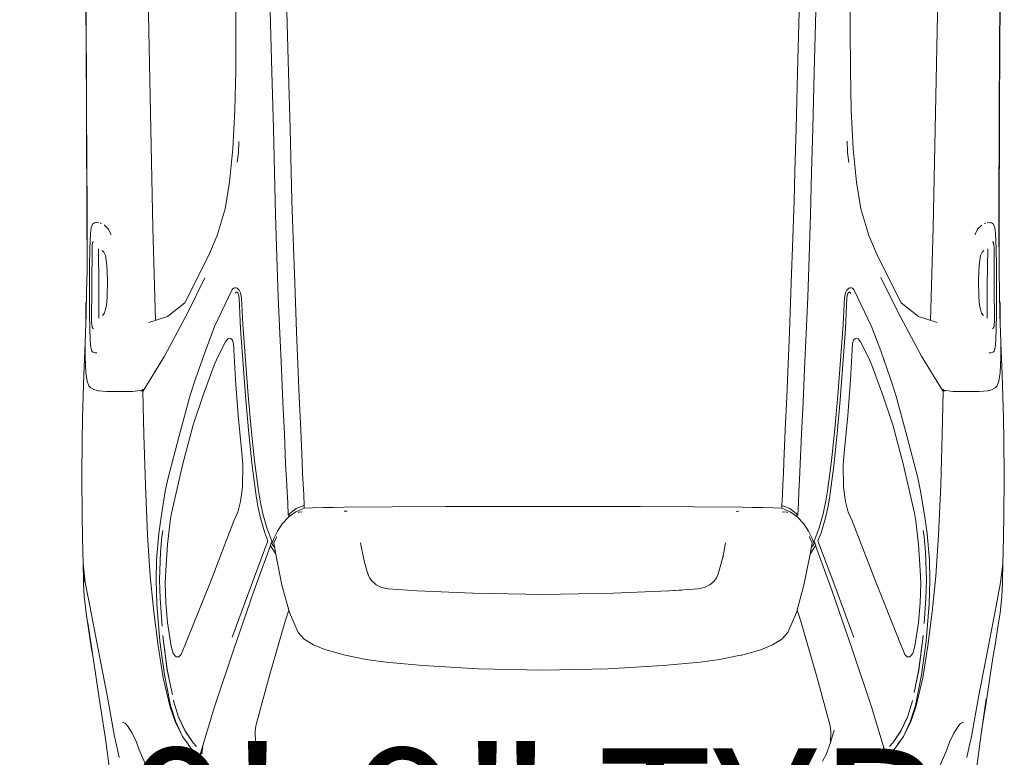
# Model space of a CAD drawing. Units: millimetres. Extents: x 595116 to 630915, y 909473 to 920225.
# Tile 115 of 134: x 629331 to 629393, y 919419 to 919466. Entities that reach past the tile are written whole.
import ezdxf

# ---------------------------------------------------------------- set-up
doc = ezdxf.new("R2010")
doc.units = ezdxf.units.MM
doc.layers.add('C-PRKG-VEHI', color=8, linetype='Continuous', lineweight=13)
doc.layers.add('Dimension', color=3, linetype='Continuous', lineweight=18)
doc.styles.get("Standard").update_dxf_attribs({"font": 'arial.ttf'})
doc.dimstyles.new('ISO-25', dxfattribs={"dimtxt": 9, "dimasz": 6, "dimexe": 1.25, "dimexo": 0.625, "dimtad": 1, "dimlunit": 4, "dimtxsty": 'Standard', "dimcen": 2.5, "dimadec": 0, "dimazin": 0, "dimtfac": 1, "dimtmove": 0, "dimatfit": 3, "dimfxl": 1, "dimarcsym": 0})

# ---------------------------------------------------------------- blocks, each defined once
blk = doc.blocks.new('A$C7ADB3080')
for p, q in [((2652.6, 1836.8), (2920.1, 1835.4)), ((2925, 1835.1), (2654.1, 1836.7)), ((3154.5, 1834.7), (2920.1, 1835.4)), ((2925, 1835.1), (3140.2, 1834.4)), ((3269.2, 1835.3), (3230.4, 1834.5)), ((3311.5, 1836.1), (3269.2, 1835.3)), ((3290.9, 1836.5), (3285.7, 1835.6)), ((3301, 1836.5), (3290.9, 1836.5)), ((3290.9, 1836.5), (3301, 1836.5)), ((3323.5, 1836.5), (3301, 1836.5)), ((3301, 1836.5), (3323.5, 1836.5)), ((3363.4, 1837.9), (3311.5, 1836.1)), ((3392, 1838.1), (3363.4, 1837.9)), ((3365.8, 1837.9), (3365.3, 1837.9)), ((3424.7, 1840.3), (3365.8, 1837.9)), ((3420.9, 1836.7), (3392, 1838.1)), ((3437.5, 1834.4), (3420.9, 1836.7)), ((3465.3, 1841.8), (3424.7, 1840.3)), ((3506.8, 1843), (3465.3, 1841.8)), ((3548.4, 1843.9), (3506.8, 1843)), ((3615.8, 1844.5), (3548.4, 1843.9)), ((3693.3, 1843.9), (3615.8, 1844.5)), ((3760.4, 1842.6), (3693.3, 1843.9)), ((3760.4, 1842.6), (3777.5, 1842)), ((3780.6, 1841.8), (3777.5, 1842)), ((3817.8, 1840.9), (3777.6, 1842)), ((3777.6, 1842), (3784.7, 1841.8)), ((3816.5, 1837.6), (3780.6, 1841.8)), ((3856.8, 1830), (3816.5, 1837.6)), ((3842, 1840.1), (3817.8, 1840.9)), ((3873.8, 1836.4), (3842, 1840.1)), ((3896.2, 1832.9), (3873.8, 1836.4)), ((3138.8, 1818), (3139.2, 1820.6)), ((3138.8, 1816.6), (3138.9, 1817.6)), ((3139.2, 1812.5), (3138.8, 1816.6)), ((3141.5, 1824), (3139.2, 1820.6)), ((3140.2, 1834.4), (3154.5, 1834.3)), ((3155.1, 1834.3), (3141.2, 1834.3)), ((3141.2, 1834.3), (3141.2, 1834.3)), ((3148.6, 1826.5), (3141.5, 1824)), ((3158.6, 1827.8), (3148.6, 1826.5)), ((3154.5, 1834.7), (3189.7, 1834.5)), ((3167.6, 1834.3), (3155.1, 1834.3)), ((3173, 1828.6), (3158.6, 1827.8)), ((3167.2, 1834.3), (3179.8, 1834.4)), ((3173, 1828.6), (3189, 1829)), ((3175.3, 1823.4), (3174.9, 1821.4)), ((3175.3, 1823.4), (3176.5, 1824)), ((3177.6, 1824.3), (3176.5, 1824)), ((3180.9, 1824.9), (3177.6, 1824.3)), ((3179.8, 1834.4), (3189.8, 1834.5)), ((3185.7, 1825.1), (3180.9, 1824.9)), ((3257.4, 1825.6), (3185.7, 1825.1)), ((3189, 1829), (3218.8, 1829.6)), ((3189.7, 1834.5), (3230.4, 1834.5)), ((3218.8, 1829.6), (3249.2, 1829.8)), ((3249.2, 1829.8), (3278.5, 1830)), ((3325.3, 1825.8), (3257.4, 1825.6)), ((3278.5, 1830), (3294.3, 1829.9)), ((3294.3, 1829.9), (3309.6, 1829.8)), ((3309.6, 1829.8), (3338.2, 1829.4)), ((3330.2, 1825.6), (3325.3, 1825.8)), ((3334.3, 1825.1), (3330.2, 1825.6)), ((3336.4, 1824.3), (3334.3, 1825.1)), ((3334.5, 1825), (3335.7, 1824.9)), ((3335.7, 1824.9), (3337.6, 1824)), ((3337.6, 1824), (3336.4, 1824.3)), ((3337.6, 1824), (3338, 1821.8)), ((3359.1, 1828.7), (3338.2, 1829.4)), ((3368.6, 1828), (3359.1, 1828.7)), ((3376.8, 1826.8), (3368.6, 1828)), ((3380.5, 1825.5), (3376.8, 1826.8)), ((3382.5, 1823.5), (3380.5, 1825.5)), ((3383.7, 1819.1), (3382.5, 1823.5)), ((3384, 1816), (3383.7, 1819.1)), ((3445.8, 1830.9), (3437.5, 1834.4)), ((3445.8, 1830.9), (3449.9, 1827.1)), ((3449.9, 1827.1), (3453.1, 1821.8)), ((3453.1, 1821.8), (3454.9, 1815.7)), ((3938.8, 1813.9), (3856.8, 1830)), ((3896.2, 1832.9), (3937.3, 1826.5)), ((3937.3, 1826.5), (3958, 1823.1)), ((3958, 1823.1), (4042.4, 1810.1)), ((3139.6, 1808.8), (3139.6, 1809.6)), ((3140.7, 1807.1), (3139.6, 1808.8)), ((3143.9, 1801.9), (3143.8, 1801.9)), ((3151.3, 1793.8), (3143.9, 1801.9)), ((3187.9, 1813.2), (3257.6, 1812.5)), ((3194.7, 1802.6), (3191.3, 1806.1)), ((3200.5, 1799.8), (3194.7, 1802.6)), ((3218.3, 1797.4), (3200.5, 1799.8)), ((3257.6, 1812.5), (3318.7, 1812.5)), ((3301.9, 1799.5), (3294.9, 1797.7)), ((3309.3, 1801.6), (3301.9, 1799.5)), ((3313.6, 1805.2), (3309.3, 1801.6)), ((3454.9, 1815.7), (3455.1, 1815)), ((3455.1, 1815), (3455.4, 1813.2)), ((3455.4, 1813.2), (3456.9, 1797.4)), ((4032, 1795.9), (3938.8, 1813.9)), ((4110.6, 1799.9), (4035.1, 1810.4)), ((4035.2, 1810.4), (4035.1, 1810.4)), ((4042.4, 1810.1), (4096.4, 1801.8)), ((4202.8, 1787.5), (4110.6, 1799.9)), ((3160.5, 1789.8), (3151.3, 1793.8)), ((3161.6, 1789.6), (3160.5, 1789.8)), ((3247.2, 1796.1), (3218.3, 1797.4)), ((3278.4, 1796.4), (3247.2, 1796.1)), ((3294.9, 1797.7), (3278.4, 1796.4)), ((3456.9, 1797.4), (3456.9, 1768.6)), ((4106, 1782.7), (4032, 1795.9)), ((4125.1, 1778.5), (4106, 1782.7)), ((3456.9, 1768.6), (3456.9, 1748.3)), ((4080, 1765.6), (4079.5, 1767.9)), ((4081, 1763.4), (4079.8, 1766.2)), ((4082.5, 1761.6), (4081, 1763.4)), ((4086.1, 1758.5), (4082.5, 1761.6)), ((4145.5, 1773.8), (4125.1, 1778.5)), ((3454.3, 1729.9), (3456.9, 1748.3)), ((4099.9, 1749.3), (4086.1, 1758.5)), ((4116.9, 1741.3), (4099.9, 1749.3)), ((3456.6, 1729.3), (3390, 1688.5)), ((3455.3, 1729.9), (3452.5, 1730)), ((3452.6, 1726.9), (3455.5, 1729.2)), ((3455.3, 1729.2), (3455.3, 1733.4)), ((3455.3, 1728.5), (3455.3, 1729)), ((3537.8, 1727.6), (3456.6, 1729.3)), ((3632.9, 1724.7), (3537.8, 1727.6)), ((3726.9, 1720.6), (3632.9, 1724.7)), ((4131.6, 1736.2), (4116.9, 1741.3)), ((4180, 1714.9), (4131.6, 1736.2)), ((3148.3, 1710.7), (2594.2, 1721.7)), ((3323, 1705.8), (3148.3, 1710.7)), ((3327.1, 1717.9), (3315.3, 1682.8)), ((3804.6, 1715.3), (3726.9, 1720.6)), ((3871.4, 1708.8), (3804.6, 1715.3)), ((3935.4, 1700.8), (3871.4, 1708.8)), ((3390, 1688.5), (3307.9, 1644.8)), ((3644.1, 1687), (3619.1, 1681.8)), ((3619.1, 1681.8), (3644.1, 1687)), ((3689.1, 1694.4), (3644.1, 1687)), ((3644.1, 1687), (3689.1, 1694.4)), ((3724.3, 1699.5), (3689.1, 1694.4)), ((3689.1, 1694.4), (3724.3, 1699.5)), ((3718.4, 1692), (3730.4, 1693.4)), ((3774.5, 1703.9), (3724.3, 1699.5)), ((3724.3, 1699.5), (3774.5, 1703.9)), ((3730.4, 1693.4), (3759.2, 1696)), ((3759.2, 1696), (3811.2, 1697.9)), ((3812.3, 1704.6), (3774.5, 1703.9)), ((3774.5, 1703.9), (3812.3, 1704.6)), ((3793.1, 1686.4), (3817.7, 1687.2)), ((3817.7, 1687.2), (3793.1, 1686.4)), ((3811.2, 1697.9), (3846.5, 1697)), ((3856.9, 1703.3), (3812.3, 1704.6)), ((3812.3, 1704.6), (3856.9, 1703.3)), ((3817.7, 1687.2), (3854.8, 1686)), ((3854.8, 1686), (3817.7, 1687.2)), ((3846.5, 1697), (3893.4, 1693.5)), ((3926.7, 1697.5), (3856.9, 1703.3)), ((3856.9, 1703.3), (3926.7, 1697.5)), ((3916.3, 1691.8), (3917.5, 1691.7)), ((3979.7, 1683.5), (3917.3, 1691.7)), ((3917.5, 1691.7), (3981.3, 1683.4)), ((3990.3, 1688.8), (3926.7, 1697.5)), ((3926.7, 1697.5), (3990.3, 1688.8)), ((3995.6, 1690.9), (3935.4, 1700.8)), ((4048.1, 1677.1), (3990.3, 1688.8)), ((3990.3, 1688.8), (4048.1, 1677.1)), ((4050.7, 1678.1), (3995.6, 1690.9)), ((3315.3, 1682.8), (3289.8, 1650.3)), ((3619.1, 1681.8), (3540, 1661.1)), ((3540, 1661.1), (3619.1, 1681.8)), ((3592.6, 1654.4), (3685.5, 1675.3)), ((3685.5, 1675.3), (3592.6, 1654.4)), ((3685.5, 1675.3), (3701, 1677.9)), ((3701, 1677.9), (3685.5, 1675.3)), ((3701, 1677.9), (3744.9, 1682.9)), ((3744.9, 1682.9), (3701, 1677.9)), ((3744.9, 1682.9), (3793.1, 1686.4)), ((3793.1, 1686.4), (3744.9, 1682.9)), ((3854.8, 1686), (3891.3, 1682.8)), ((3891.3, 1682.8), (3854.8, 1686)), ((3891.3, 1682.8), (3936.2, 1676.3)), ((3936.2, 1676.3), (3891.3, 1682.8)), ((3936.2, 1676.3), (3950.2, 1672.4)), ((3950.2, 1672.4), (3936.2, 1676.3)), ((3950.2, 1672.4), (3956.1, 1666.6)), ((3956.1, 1666.6), (3950.2, 1672.4)), ((4004.3, 1678.6), (3979.7, 1683.5)), ((3981.3, 1683.4), (4023.5, 1674.8)), ((4010.7, 1677.4), (4004.3, 1678.6)), ((4038.4, 1671.7), (4039.3, 1671.5)), ((4039.3, 1671.5), (4069.8, 1662)), ((4078.8, 1667.3), (4048.1, 1677.1)), ((4048.1, 1677.1), (4078.8, 1667.3)), ((4050.7, 1678.1), (4080.1, 1667.8)), ((4050.7, 1678.1), (4050.7, 1678.1)), ((4080.1, 1667.8), (4050.7, 1678.1)), ((3289.8, 1650.3), (3201.4, 1606)), ((3540, 1661.1), (3463.8, 1640.1)), ((3463.8, 1640.1), (3540, 1661.1)), ((3519.3, 1634.8), (3592.6, 1654.4)), ((3592.6, 1654.4), (3519.3, 1634.8)), ((3951.6, 1657.2), (3925.2, 1646.4)), ((3925.2, 1646.4), (3951.6, 1657.2)), ((3956, 1661.6), (3951.6, 1657.2)), ((3951.6, 1657.2), (3956, 1661.6)), ((3956.1, 1666.6), (3956, 1661.6)), ((3956, 1661.6), (3956.1, 1666.6)), ((4095.5, 1649.7), (4069.3, 1662.1)), ((4069.8, 1662), (4096.4, 1649.5)), ((4106, 1654.5), (4078.8, 1667.3)), ((4078.8, 1667.3), (4106, 1654.5)), ((4080.1, 1667.8), (4106, 1654.5)), ((4106, 1654.5), (4080.1, 1667.8)), ((4117.9, 1634.7), (4095.5, 1649.7)), ((4096.4, 1649.5), (4118.4, 1634.8)), ((4121, 1644.1), (4106, 1654.5)), ((4106, 1654.5), (4120.9, 1644.2)), ((3307.9, 1644.8), (3242.4, 1612.3)), ((3463.8, 1640.1), (3431.3, 1629.6)), ((3431.3, 1629.6), (3463.8, 1640.1)), ((3463.6, 1615.6), (3519.3, 1634.8)), ((3519.3, 1634.8), (3463.6, 1615.6)), ((3925.2, 1646.4), (3817.2, 1603)), ((3817.2, 1603), (3925.2, 1646.4)), ((4125.2, 1628.3), (4117.9, 1634.7)), ((4118.4, 1634.8), (4125.2, 1628.5)), ((4120.9, 1644.2), (4121.2, 1644)), ((4128, 1639.3), (4121.3, 1643.9)), ((4136.9, 1631), (4128, 1639.3)), ((4134.8, 1633), (4134.9, 1633)), ((4134.9, 1633), (4145.3, 1623.3)), ((4145.3, 1623.3), (4136.9, 1631)), ((3431.3, 1629.6), (3380.1, 1611.8)), ((3380.1, 1611.8), (3431.3, 1629.6)), ((3407.4, 1595.4), (3463.6, 1615.6)), ((3463.6, 1615.6), (3407.4, 1595.4)), ((4050.4, 1594.4), (4142.2, 1622)), ((4138.6, 1618.2), (4124.8, 1616.8)), ((4125.2, 1628.5), (4125, 1628.4)), ((4139.4, 1620.9), (4137.7, 1619.3)), ((4138.9, 1617.7), (4137.7, 1619.3)), ((4146.3, 1623.6), (4139.4, 1620.9)), ((4140.8, 1621.4), (4140.7, 1621.5)), ((3201.4, 1606), (3163.1, 1589.7)), ((3334.6, 1594.5), (3264.7, 1561.2)), ((3264.7, 1561.2), (3334.6, 1594.5)), ((3380.1, 1611.8), (3334.6, 1594.5)), ((3334.6, 1594.5), (3380.1, 1611.8)), ((3392.8, 1588.9), (3407.4, 1595.4)), ((3407.4, 1595.4), (3392.8, 1588.9)), ((3817.2, 1603), (3700.4, 1558.4)), ((3700.4, 1558.4), (3817.2, 1603)), ((3941.5, 1558.3), (4050.4, 1594.4)), ((3163.1, 1589.7), (3112.6, 1574.6)), ((3363.1, 1573.8), (3392.8, 1588.9)), ((3392.8, 1588.9), (3363.1, 1573.8)), ((2999.6, 1560.1), (2926.8, 1556.4)), ((3062.7, 1566.3), (2999.6, 1560.1)), ((3112.6, 1574.6), (3062.7, 1566.3)), ((3262.5, 1558.7), (3261.6, 1556.1)), ((3261.6, 1556.1), (3262.5, 1558.7)), ((3264.7, 1561.2), (3262.5, 1558.7)), ((3262.5, 1558.7), (3264.7, 1561.2)), ((3356.4, 1565.7), (3357.5, 1569.1)), ((3357.5, 1569.1), (3356.4, 1565.7)), ((3357.6, 1563.2), (3356.4, 1565.7)), ((3356.4, 1565.7), (3357.6, 1563.2)), ((3357.5, 1569.1), (3363.1, 1573.8)), ((3363.1, 1573.8), (3357.5, 1569.1)), ((3360.3, 1560.6), (3357.6, 1563.2)), ((3357.6, 1563.2), (3360.3, 1560.6)), ((3364.2, 1559.4), (3360.3, 1560.6)), ((3360.3, 1560.6), (3360.8, 1560.5)), ((3360.3, 1560.6), (3364.2, 1559.4)), ((3366.9, 1559), (3364.2, 1559.4)), ((3364.2, 1559.4), (3366.9, 1559)), ((3366.7, 1559.1), (3366.9, 1559)), ((3434.5, 1554.7), (3366.9, 1559)), ((3366.9, 1559), (3434.5, 1554.7)), ((3700.4, 1558.4), (3683.7, 1550.7)), ((3683.7, 1550.7), (3700.4, 1558.4)), ((3919.8, 1561.3), (3822.4, 1525.6)), ((3832.9, 1520.5), (3941.5, 1558.3)), ((2773, 1554.3), (2622.6, 1554.3)), ((2851.6, 1554.7), (2773, 1554.3)), ((2926.8, 1556.4), (2851.6, 1554.7)), ((3006.7, 1549.4), (2985.7, 1548.6)), ((3025.6, 1551.6), (3006.7, 1549.4)), ((3261.6, 1556.1), (3261.6, 1553.9)), ((3261.6, 1553.9), (3261.6, 1556.1)), ((3261.6, 1556.1), (3261.6, 1555.9)), ((3261.6, 1553.9), (3262.3, 1551.6)), ((3262.3, 1551.6), (3261.6, 1553.9)), ((3262.2, 1551.8), (3262.3, 1551.6)), ((3262.3, 1551.6), (3265.7, 1548.2)), ((3265.7, 1548.2), (3262.3, 1551.6)), ((3265.7, 1548.2), (3271, 1545.4)), ((3271, 1545.4), (3265.7, 1548.2)), ((3271, 1550.8), (3269.2, 1553.1)), ((3269.5, 1552.8), (3269.6, 1553.9)), ((3269.6, 1553.9), (3272.3, 1555.5)), ((3274.3, 1549.1), (3271, 1550.8)), ((3271, 1545.4), (3280.2, 1543.8)), ((3280.2, 1543.8), (3271, 1545.4)), ((3280.2, 1548.2), (3274.3, 1549.1)), ((3338.5, 1545.3), (3280.2, 1548.2)), ((3280.2, 1543.8), (3330.4, 1541.1)), ((3330.4, 1541.1), (3280.2, 1543.8)), ((3330.4, 1541.1), (3397.7, 1536.4)), ((3397.7, 1536.4), (3330.4, 1541.1)), ((3405.7, 1540.6), (3338.5, 1545.3)), ((3472.6, 1535.6), (3405.7, 1540.6)), ((3501.9, 1549.7), (3434.5, 1554.7)), ((3434.5, 1554.7), (3501.9, 1549.7)), ((3566, 1543.9), (3501.9, 1549.7)), ((3501.9, 1549.7), (3566, 1543.9)), ((3594.2, 1541.4), (3566, 1543.9)), ((3566, 1543.9), (3594.2, 1541.4)), ((3636.8, 1542), (3594.2, 1541.4)), ((3594.2, 1541.4), (3636.8, 1542)), ((3664.1, 1545.3), (3636.8, 1542)), ((3636.8, 1542), (3664.1, 1545.3)), ((3683.7, 1550.7), (3664.1, 1545.3)), ((3664.1, 1545.3), (3683.7, 1550.7)), ((3397.7, 1536.4), (3464.1, 1531.2)), ((3464.1, 1531.2), (3397.7, 1536.4)), ((3464.1, 1531.2), (3527.2, 1525.6)), ((3527.2, 1525.6), (3464.1, 1531.2)), ((3536, 1530), (3472.6, 1535.6)), ((3527.2, 1525.6), (3587, 1519.2)), ((3587, 1519.2), (3527.2, 1525.6)), ((3596.5, 1523.8), (3536, 1530)), ((3653.1, 1515.9), (3596.5, 1523.8)), ((3822.4, 1525.6), (3738.1, 1493.8)), ((3746.6, 1489.3), (3832.9, 1520.5)), ((4094.2, 1524.4), (4096.2, 1523.8)), ((4094.2, 1524.4), (4117.8, 1517.2)), ((3587, 1519.2), (3643.8, 1511.6)), ((3643.8, 1511.6), (3587, 1519.2)), ((3643.8, 1511.6), (3662.7, 1508.4)), ((3662.7, 1508.4), (3643.8, 1511.6)), ((3672.4, 1512.7), (3653.1, 1515.9)), ((3662.7, 1508.4), (3687.1, 1503.5)), ((3687.1, 1503.5), (3662.7, 1508.4)), ((3696.9, 1507.4), (3672.4, 1512.7)), ((3687.1, 1503.5), (3713.6, 1496.2)), ((3713.6, 1496.2), (3687.1, 1503.5)), ((3723.1, 1499.8), (3696.9, 1507.4)), ((3991.5, 1490.9), (4085.9, 1517)), ((4085.9, 1517), (3991.5, 1490.9)), ((4085.9, 1517), (4096.8, 1518.2)), ((4096.8, 1518.2), (4085.9, 1517)), ((4096.8, 1518.2), (4117.8, 1517.2)), ((4117.8, 1517.2), (4096.8, 1518.2)), ((4117.8, 1517.2), (4140.4, 1509.4)), ((4140.4, 1509.4), (4117.8, 1517.2)), ((4140.4, 1509.4), (4152.4, 1502.3)), ((4152.4, 1502.3), (4140.4, 1509.4)), ((2855.6, 1486.9), (2739.8, 1490)), ((2739.8, 1490), (2855.6, 1486.9)), ((2961.5, 1483.8), (2855.6, 1486.9)), ((2855.6, 1486.9), (2961.5, 1483.8)), ((3043.6, 1481.5), (2961.5, 1483.8)), ((2961.5, 1483.8), (3043.6, 1481.5)), ((3713.6, 1496.2), (3716.2, 1495.2)), ((3738.7, 1486.4), (3713.6, 1496.2)), ((3738.1, 1493.8), (3723.1, 1499.8)), ((3741.7, 1483.1), (3730.8, 1477.9)), ((3743.8, 1486.4), (3733.7, 1482.6)), ((3736.9, 1487.1), (3738.7, 1486.4)), ((3738.2, 1493.8), (3738.1, 1493.8)), ((3746.3, 1489.5), (3738.5, 1486.3)), ((3738.5, 1486.3), (3739.1, 1484.6)), ((3738.7, 1486.4), (3740.1, 1486.9)), ((3738.7, 1486.3), (3738.7, 1486.4)), ((3738.7, 1484.5), (3738.7, 1485.8)), ((3748.7, 1481.8), (3741.7, 1483.1)), ((3749.9, 1481.6), (3743.8, 1486.4)), ((3746.3, 1489.5), (3762, 1479.9)), ((3887, 1461.1), (3991.5, 1490.9)), ((3991.5, 1490.9), (3887, 1461.1)), ((3123.9, 1479.4), (3043.6, 1481.5)), ((3043.6, 1481.5), (3123.9, 1479.4)), ((3203.4, 1477), (3123.9, 1479.4)), ((3123.9, 1479.4), (3203.4, 1477)), ((3279, 1474.4), (3203.4, 1477)), ((3203.4, 1477), (3279, 1474.4)), ((3347.7, 1471.6), (3279, 1474.4)), ((3279, 1474.4), (3347.7, 1471.6)), ((3413.9, 1468.6), (3347.7, 1471.6)), ((3347.7, 1471.6), (3413.9, 1468.6)), ((3476.6, 1465.7), (3413.9, 1468.6)), ((3413.9, 1468.6), (3476.6, 1465.7)), ((3536.4, 1463), (3476.6, 1465.7)), ((3476.6, 1465.7), (3536.4, 1463)), ((3706.1, 1467), (3692.8, 1454.4)), ((3719.7, 1476), (3706.1, 1467)), ((3733.7, 1482.6), (3719.7, 1476)), ((3730.8, 1477.9), (3730, 1477.5)), ((3755.7, 1480.5), (3748.7, 1481.8)), ((3762.8, 1479.3), (3755.7, 1480.5)), ((3762, 1479.9), (3762.7, 1479.3)), ((3821.6, 1467.4), (3762.8, 1479.3)), ((3872.7, 1453.3), (3821.6, 1467.4)), ((2740.5, 1458.5), (2856, 1455.4)), ((2856, 1455.4), (2740.5, 1458.5)), ((2856, 1455.4), (2961.6, 1452.4)), ((2961.6, 1452.4), (2856, 1455.4)), ((2961.6, 1452.4), (3043.5, 1450.2)), ((3043.5, 1450.2), (2961.6, 1452.4)), ((3043.5, 1450.2), (3097.4, 1448.7)), ((3097.4, 1448.7), (3043.5, 1450.2)), ((3097.4, 1448.7), (3168.2, 1446.4)), ((3168.2, 1446.4), (3097.4, 1448.7)), ((3168.2, 1446.4), (3252, 1443.4)), ((3252, 1443.4), (3168.2, 1446.4)), ((3593.8, 1460.5), (3536.4, 1463)), ((3536.4, 1463), (3593.8, 1460.5)), ((3622.3, 1459.2), (3593.8, 1460.5)), ((3593.8, 1460.5), (3622.3, 1459.2)), ((3645.7, 1457.9), (3622.3, 1459.2)), ((3622.3, 1459.2), (3645.7, 1457.9)), ((3666.9, 1456.8), (3645.7, 1457.9)), ((3645.7, 1457.9), (3666.9, 1456.8)), ((3688.7, 1455.7), (3666.9, 1456.8)), ((3666.9, 1456.8), (3688.7, 1455.7)), ((3677.3, 1440.6), (3688.7, 1455.7)), ((3692.8, 1454.4), (3683.5, 1441.6)), ((3688.7, 1453.7), (3687.2, 1453.8)), ((3688.7, 1455.7), (3691.7, 1452.8)), ((3689.8, 1454.7), (3688.7, 1453.7)), ((3868.3, 1454.5), (3887, 1461.1)), ((3887, 1461.1), (3868.3, 1454.5)), ((3910.3, 1437.3), (3872.7, 1453.3)), ((3252, 1443.4), (3344.7, 1439.9)), ((3344.7, 1439.9), (3252, 1443.4)), ((3344.7, 1439.9), (3405.5, 1437.5)), ((3405.5, 1437.5), (3344.7, 1439.9)), ((3405.5, 1437.5), (3467.2, 1434.9)), ((3467.2, 1434.9), (3405.5, 1437.5)), ((3467.2, 1434.9), (3528.9, 1432.2)), ((3528.9, 1432.2), (3467.2, 1434.9)), ((3528.9, 1432.2), (3589.5, 1429.6)), ((3589.5, 1429.6), (3528.9, 1432.2)), ((3589.5, 1429.6), (3610.4, 1428.6)), ((3610.4, 1428.6), (3589.5, 1429.6)), ((3610.4, 1428.6), (3631.1, 1427.6)), ((3631.1, 1427.6), (3610.4, 1428.6)), ((3631.1, 1427.6), (3651.3, 1426.7)), ((3651.3, 1426.7), (3631.1, 1427.6)), ((3671.3, 1425.7), (3677.3, 1440.6)), ((3683.5, 1441.6), (3676.4, 1425.7)), ((3683.8, 1435.6), (3683.3, 1426.1)), ((3684.4, 1437.3), (3683.8, 1435.6)), ((3923.1, 1425.6), (3910.3, 1437.3)), ((3651.3, 1426.7), (3671.3, 1425.7)), ((3671.3, 1425.7), (3651.3, 1426.7)), ((3676.4, 1425.9), (3671.3, 1425.7)), ((3675.9, 1409.8), (3675.4, 1390)), ((3676.4, 1425.7), (3675.9, 1409.8)), ((3933.8, 1407.9), (3923.1, 1425.6)), ((3675.4, 1390), (3675.1, 1370.7)), ((3942.9, 1386), (3933.8, 1407.9)), ((3953.5, 1347.9), (3942.9, 1386)), ((3675.1, 1370.7), (3674.7, 1351.3)), ((3674.7, 1351.3), (3673.7, 1260.2)), ((3682.1, 1344.7), (3682.8, 1339.8)), ((3961.1, 1308.5), (3953.3, 1347.8)), ((3770, 1314.4), (3741.9, 1319.7)), ((3775.6, 1312.9), (3765.8, 1315.1)), ((3794, 1307.7), (3775.6, 1312.9)), ((3801.6, 1305.4), (3794, 1307.7)), ((3807.7, 1302.5), (3801.6, 1305.4)), ((3813.6, 1298.2), (3807.7, 1302.5)), ((3820.8, 1290.2), (3813.6, 1298.2)), ((3966.3, 1272), (3961.1, 1308.5)), ((3820.9, 1289.8), (3818.1, 1293.1)), ((3825.7, 1280.1), (3820.9, 1289.8)), ((3828.2, 1267.8), (3825.7, 1280.1)), ((3832.1, 1214), (3828.2, 1267.8)), ((3972.7, 1202.5), (3966.3, 1272)), ((3673.7, 1260.2), (3673.2, 1159.8)), ((3832, 1212.9), (3830.5, 1236.6)), ((3836.6, 1108.1), (3832, 1212.9)), ((3978.7, 1098.1), (3972.7, 1202.5)), ((3673.2, 1159.8), (3673.1, 1061.9)), ((3838.8, 976.2), (3836.6, 1108.1)), ((3981.5, 976.2), (3978.7, 1098.1)), ((3673.1, 1061.9), (3673.4, 976.2)), ((3673.4, 976.2), (3673.1, 890.5)), ((3836.6, 844.3), (3838.8, 976.2)), ((3978.7, 854.2), (3981.5, 976.2)), ((3673.1, 890.5), (3673.2, 792.6)), ((3972.7, 749.9), (3978.7, 854.2)), ((3832, 739.5), (3836.6, 844.3)), ((3673.2, 792.6), (3673.7, 692.2)), ((3966.3, 680.4), (3972.7, 749.9)), ((3828.2, 684.6), (3832, 739.5)), ((3673.7, 692.2), (3674.7, 601.1)), ((3820.7, 662), (3825.6, 672.2)), ((3825.6, 672.2), (3828.2, 684.6)), ((3961, 643.5), (3966.3, 680.4)), ((3800.8, 646.4), (3807.5, 649.8)), ((3801.5, 647), (3806, 649)), ((3807.5, 649.8), (3813.4, 654)), ((3813.4, 654), (3820.8, 662.4)), ((3741.9, 632.7), (3775.6, 639.5)), ((3775.6, 639.5), (3794, 644.6)), ((3794, 644.6), (3801.5, 647)), ((3953.3, 603.8), (3961, 643.5)), ((3674.7, 601.1), (3675.1, 581.7)), ((3682.1, 607.7), (3682.1, 601.7)), ((3942.5, 565.4), (3953.3, 603.8)), ((3675.1, 581.7), (3675.4, 562.4)), ((3675.4, 562.4), (3675.9, 542.6)), ((3933.6, 543.9), (3942.5, 565.4)), ((3675.9, 542.6), (3676.4, 526.7)), ((3922.9, 526.5), (3933.6, 543.9)), ((3528.9, 520.1), (3467.2, 517.5)), ((3467.2, 517.5), (3528.9, 520.1)), ((3589.5, 522.8), (3528.9, 520.1)), ((3528.9, 520.1), (3589.5, 522.8)), ((3610.4, 523.8), (3589.5, 522.8)), ((3589.5, 522.8), (3610.4, 523.8)), ((3631.1, 524.7), (3610.4, 523.8)), ((3610.4, 523.8), (3631.1, 524.7)), ((3651.3, 525.7), (3631.1, 524.7)), ((3631.1, 524.7), (3651.3, 525.7)), ((3671.3, 526.7), (3651.3, 525.7)), ((3651.3, 525.7), (3671.3, 526.7)), ((3677.3, 511.8), (3671.3, 526.7)), ((3671.3, 526.7), (3676.4, 526.5)), ((3676.4, 526.7), (3683.5, 510.8)), ((3683.5, 522.6), (3683.8, 516.7)), ((3910.3, 515.1), (3922.9, 526.5)), ((3043.5, 502.2), (2961.6, 500)), ((2961.6, 500), (3043.5, 502.2)), ((3097.4, 503.7), (3043.5, 502.2)), ((3043.5, 502.2), (3097.4, 503.7)), ((3168.2, 506), (3097.4, 503.7)), ((3097.4, 503.7), (3168.2, 506)), ((3252, 509), (3168.2, 506)), ((3168.2, 506), (3252, 509)), ((3344.7, 512.5), (3252, 509)), ((3252, 509), (3344.7, 512.5)), ((3405.5, 514.9), (3344.7, 512.5)), ((3344.7, 512.5), (3405.5, 514.9)), ((3467.2, 517.5), (3405.5, 514.9)), ((3405.5, 514.9), (3467.2, 517.5)), ((3688.7, 496.6), (3677.3, 511.8)), ((3683.5, 510.8), (3692.8, 498)), ((3683.8, 516.7), (3684.4, 515.1)), ((3872.7, 499.1), (3910.3, 515.1)), ((2856, 496.9), (2740.5, 493.9)), ((2740.5, 493.9), (2856, 496.9)), ((2961.6, 500), (2856, 496.9)), ((2856, 496.9), (2961.6, 500)), ((3347.7, 480.8), (3413.9, 483.8)), ((3413.9, 483.8), (3347.7, 480.8)), ((3413.9, 483.8), (3476.6, 486.7)), ((3476.6, 486.7), (3413.9, 483.8)), ((3476.6, 486.7), (3536.4, 489.3)), ((3536.4, 489.3), (3476.6, 486.7)), ((3536.4, 489.3), (3593.8, 491.8)), ((3593.8, 491.8), (3536.4, 489.3)), ((3593.8, 491.8), (3622.3, 493.2)), ((3622.3, 493.2), (3593.8, 491.8)), ((3622.3, 493.2), (3645.7, 494.4)), ((3645.7, 494.4), (3622.3, 493.2)), ((3645.7, 494.4), (3666.9, 495.6)), ((3666.9, 495.6), (3645.7, 494.4)), ((3666.9, 495.6), (3688.7, 496.6)), ((3688.7, 496.6), (3666.9, 495.6)), ((3687.2, 498.6), (3688.7, 498.7)), ((3691.7, 499.6), (3688.7, 496.6)), ((3688.7, 498.7), (3689.8, 497.7)), ((3692.8, 498), (3706.1, 485.3)), ((3706.1, 485.3), (3719.7, 476.4)), ((3762.8, 473.1), (3821.6, 484.9)), ((3821.6, 484.9), (3872.7, 499.1)), ((3887, 491.2), (3868.3, 497.9)), ((3868.3, 497.9), (3887, 491.2)), ((3991.5, 461.4), (3887, 491.2)), ((3887, 491.2), (3991.5, 461.4)), ((2739.8, 462.4), (2855.6, 465.5)), ((2855.6, 465.5), (2739.8, 462.4)), ((2855.6, 465.5), (2961.5, 468.6)), ((2961.5, 468.6), (2855.6, 465.5)), ((2961.5, 468.6), (3043.6, 470.9)), ((3043.6, 470.9), (2961.5, 468.6)), ((3043.6, 470.9), (3123.9, 472.9)), ((3123.9, 472.9), (3043.6, 470.9)), ((3123.9, 472.9), (3203.4, 475.3)), ((3203.4, 475.3), (3123.9, 472.9)), ((3203.4, 475.3), (3279, 478)), ((3279, 478), (3203.4, 475.3)), ((3279, 478), (3347.7, 480.8)), ((3347.7, 480.8), (3279, 478)), ((3713.6, 456.1), (3738.7, 466)), ((3719.7, 476.4), (3733.7, 469.8)), ((3738.7, 466), (3728.7, 462.1)), ((3730.6, 474.5), (3730.8, 474.4)), ((3730.8, 474.4), (3741.7, 469.3)), ((3733.7, 469.8), (3743.8, 466)), ((3739.1, 467.8), (3738.5, 466.1)), ((3738.5, 466.1), (3746.3, 462.9)), ((3738.7, 466.5), (3738.7, 467.9)), ((3739.5, 465.7), (3738.7, 466)), ((3738.7, 466), (3738.7, 466)), ((3741.7, 469.3), (3748.7, 470.5)), ((3743.8, 466), (3749.9, 470.8)), ((3762, 472.5), (3746.3, 462.9)), ((3748.7, 470.5), (3755.7, 471.8)), ((3755.7, 471.8), (3762.8, 473.1)), ((3762.7, 473.1), (3762, 472.5)), ((3687.1, 448.9), (3662.7, 443.9)), ((3662.7, 443.9), (3687.1, 448.9)), ((3672.4, 439.7), (3696.9, 445)), ((3713.6, 456.1), (3687.1, 448.9)), ((3687.1, 448.9), (3713.6, 456.1)), ((3696.9, 445), (3723.1, 452.6)), ((3728.7, 462.1), (3713.6, 456.1)), ((3723.1, 452.6), (3738.1, 458.5)), ((3738.1, 458.5), (3822.4, 426.8)), ((3832.9, 431.9), (3746.7, 463.1)), ((4085.9, 435.4), (3991.5, 461.4)), ((3991.5, 461.4), (4085.9, 435.4)), ((4152.4, 450), (4140.4, 443)), ((4140.4, 443), (4152.4, 450)), ((3527.2, 426.8), (3464.1, 421.2)), ((3464.1, 421.2), (3527.2, 426.8)), ((3587, 433.2), (3527.2, 426.8)), ((3527.2, 426.8), (3587, 433.2)), ((3536, 422.4), (3596.5, 428.6)), ((3643.8, 440.8), (3587, 433.2)), ((3587, 433.2), (3643.8, 440.8)), ((3596.5, 428.6), (3653.1, 436.5)), ((3662.7, 443.9), (3643.8, 440.8)), ((3643.8, 440.8), (3662.7, 443.9)), ((3653.1, 436.5), (3672.4, 439.7)), ((3822.4, 426.8), (3919.4, 391.3)), ((3941.5, 394), (3832.9, 431.9)), ((4096.8, 434.1), (4085.9, 435.4)), ((4085.9, 435.4), (4096.8, 434.1)), ((4117.8, 435.1), (4096.8, 434.1)), ((4096.8, 434.1), (4117.8, 435.1)), ((4140.4, 443), (4117.8, 435.1)), ((4117.8, 435.1), (4140.4, 443)), ((3280.2, 408.6), (3271, 407)), ((3271, 407), (3280.2, 408.6)), ((3330.4, 411.2), (3280.2, 408.6)), ((3280.2, 408.6), (3330.4, 411.2)), ((3397.7, 415.9), (3330.4, 411.2)), ((3330.4, 411.2), (3397.7, 415.9)), ((3338.5, 407.1), (3405.7, 411.7)), ((3464.1, 421.2), (3397.7, 415.9)), ((3397.7, 415.9), (3464.1, 421.2)), ((3405.7, 411.7), (3472.6, 416.8)), ((3472.6, 416.8), (3536, 422.4)), ((3501.9, 402.7), (3566, 408.5)), ((3566, 408.5), (3501.9, 402.7)), ((3566, 408.5), (3594.2, 410.9)), ((3594.2, 410.9), (3566, 408.5)), ((3594.2, 410.9), (3636.8, 410.4)), ((3636.8, 410.4), (3594.2, 410.9)), ((3636.8, 410.4), (3664.1, 407.1)), ((3664.1, 407.1), (3636.8, 410.4)), ((2622.6, 398.1), (2773, 398.1)), ((2773, 398.1), (2851.6, 397.7)), ((2851.6, 397.7), (2926.8, 396)), ((2926.8, 396), (2999.6, 392.2)), ((2986.1, 403.8), (3006.7, 402.9)), ((2999.6, 392.2), (3062.7, 386.1)), ((3006.7, 402.9), (3025.1, 400.8)), ((3262.3, 400.8), (3261.6, 398.5)), ((3261.6, 398.5), (3262.3, 400.8)), ((3261.6, 398.5), (3261.6, 396.3)), ((3261.6, 396.3), (3261.6, 398.5)), ((3261.6, 396.4), (3261.6, 396.3)), ((3261.6, 396.3), (3262.5, 393.6)), ((3262.5, 393.6), (3261.6, 396.3)), ((3262.3, 400.8), (3262.2, 400.6)), ((3265.7, 404.2), (3262.3, 400.8)), ((3262.3, 400.8), (3265.7, 404.2)), ((3262.5, 393.6), (3264.7, 391.1)), ((3264.7, 391.1), (3262.5, 393.6)), ((3264.7, 391.1), (3334.6, 357.8)), ((3334.6, 357.8), (3264.7, 391.1)), ((3271, 407), (3265.7, 404.2)), ((3265.7, 404.2), (3271, 407)), ((3269.2, 399.3), (3271, 401.5)), ((3269.6, 398.5), (3269.5, 399.6)), ((3271.9, 397.1), (3269.6, 398.5)), ((3271, 401.5), (3274.3, 403.3)), ((3274.3, 403.3), (3280.2, 404.2)), ((3280.2, 404.2), (3338.5, 407.1)), ((3357.6, 389.2), (3360.3, 391.7)), ((3360.3, 391.7), (3357.6, 389.2)), ((3360.3, 391.7), (3364.2, 393)), ((3364.2, 393), (3360.3, 391.7)), ((3361.1, 391.9), (3360.3, 391.7)), ((3364.2, 393), (3366.9, 393.4)), ((3366.9, 393.4), (3364.2, 393)), ((3366.9, 393.4), (3366.5, 393.3)), ((3366.9, 393.4), (3434.5, 397.6)), ((3434.5, 397.6), (3366.9, 393.4)), ((3434.5, 397.6), (3501.9, 402.7)), ((3501.9, 402.7), (3434.5, 397.6)), ((3664.1, 407.1), (3683.7, 401.7)), ((3683.7, 401.7), (3664.1, 407.1)), ((3683.7, 401.7), (3700.4, 394)), ((3700.4, 394), (3683.7, 401.7)), ((3700.4, 394), (3817.2, 349.4)), ((3817.2, 349.4), (3700.4, 394)), ((4050.4, 358), (3941.5, 394)), ((3062.7, 386.1), (3112.6, 377.8)), ((3112.6, 377.8), (3163.1, 362.7)), ((3356.4, 386.7), (3357.6, 389.2)), ((3357.6, 389.2), (3356.4, 386.7)), ((3357.5, 383.2), (3356.4, 386.7)), ((3356.4, 386.7), (3357.5, 383.2)), ((3363.1, 378.6), (3357.5, 383.2)), ((3357.5, 383.2), (3363.1, 378.6)), ((3392.8, 363.5), (3363.1, 378.6)), ((3363.1, 378.6), (3392.8, 363.5)), ((3163.1, 362.7), (3201.4, 346.4)), ((3334.6, 357.8), (3380.1, 340.6)), ((3380.1, 340.6), (3334.6, 357.8)), ((3407.4, 357), (3392.8, 363.5)), ((3392.8, 363.5), (3407.4, 357)), ((3463.6, 336.8), (3407.4, 357)), ((3407.4, 357), (3463.6, 336.8)), ((4142, 330.4), (4050.4, 358)), ((3201.4, 346.4), (3289.8, 302.1)), ((3242.7, 339.9), (3307.9, 307.6)), ((3380.1, 340.6), (3431.3, 322.8)), ((3431.3, 322.8), (3380.1, 340.6)), ((3519.3, 317.6), (3463.6, 336.8)), ((3463.6, 336.8), (3519.3, 317.6)), ((3817.2, 349.4), (3925.2, 306)), ((3925.2, 306), (3817.2, 349.4)), ((4125, 335.6), (4138.5, 334.1)), ((4137.7, 333.1), (4138.9, 334.6)), ((3431.3, 322.8), (3463.8, 312.3)), ((3463.8, 312.3), (3431.3, 322.8)), ((3592.6, 298), (3519.3, 317.6)), ((3519.3, 317.6), (3592.6, 298)), ((4095.5, 302.7), (4117.9, 317.7)), ((4118.4, 317.6), (4096.4, 302.9)), ((4117.9, 317.7), (4125.2, 324.1)), ((4125.2, 323.9), (4118.4, 317.6)), ((4125, 323.9), (4125.2, 323.9)), ((4128, 313.1), (4136.9, 321.3)), ((4134.9, 319.4), (4134.8, 319.4)), ((4145.3, 329.1), (4134.9, 319.4)), ((4136.9, 321.3), (4145.3, 329.1)), ((4137.7, 333.1), (4139.4, 331.5)), ((4139.4, 331.5), (4146.3, 328.7)), ((4140.7, 330.9), (4140.8, 330.9)), ((3289.8, 302.1), (3315.3, 269.6)), ((3307.9, 307.6), (3390, 263.8)), ((3463.8, 312.3), (3540, 291.3)), ((3540, 291.3), (3463.8, 312.3)), ((3685.5, 277), (3592.6, 298)), ((3592.6, 298), (3685.5, 277)), ((3925.2, 306), (3951.6, 295.2)), ((3951.6, 295.2), (3925.2, 306)), ((4069.4, 290.3), (4095.5, 302.7)), ((4096.4, 302.9), (4069.8, 290.4)), ((4078.8, 285.1), (4106, 297.8)), ((4106, 297.8), (4078.8, 285.1)), ((4080.1, 284.6), (4106, 297.8)), ((4106, 297.8), (4080.1, 284.6)), ((4120.9, 308.2), (4106, 297.8)), ((4106, 297.8), (4109.2, 300.1)), ((4121.1, 308.3), (4120.9, 308.2)), ((4121.2, 308.4), (4128, 313.1)), ((3540, 291.3), (3619.1, 270.6)), ((3619.1, 270.6), (3540, 291.3)), ((3950.2, 280), (3936.2, 276.1)), ((3936.2, 276.1), (3950.2, 280)), ((3956.1, 285.8), (3950.2, 280)), ((3950.2, 280), (3956.1, 285.8)), ((3951.6, 295.2), (3956, 290.8)), ((3956, 290.8), (3951.6, 295.2)), ((3956, 290.8), (3956.1, 285.8)), ((3956.1, 285.8), (3956, 290.8)), ((4027.9, 278.5), (3981.3, 269)), ((4039.3, 280.8), (4038.1, 280.6)), ((4039.2, 280.8), (4041.7, 281.6)), ((4069.8, 290.4), (4039.3, 280.8)), ((4048.1, 275.3), (4078.8, 285.1)), ((4078.8, 285.1), (4048.1, 275.3)), ((4050.7, 274.3), (4080.1, 284.6)), ((4080.1, 284.6), (4050.7, 274.3)), ((3315.3, 269.6), (3327.1, 234.4)), ((3390, 263.8), (3456.6, 223)), ((3619.1, 270.6), (3644.1, 265.3)), ((3644.1, 265.3), (3619.1, 270.6)), ((3644.1, 265.3), (3689.1, 258)), ((3689.1, 258), (3644.1, 265.3)), ((3701, 274.5), (3685.5, 277)), ((3685.5, 277), (3701, 274.5)), ((3744.9, 269.5), (3701, 274.5)), ((3701, 274.5), (3744.9, 269.5)), ((3730.4, 259), (3718.4, 260.4)), ((3793.1, 266), (3744.9, 269.5)), ((3744.9, 269.5), (3793.1, 266)), ((3817.7, 265.2), (3793.1, 266)), ((3793.1, 266), (3817.7, 265.2)), ((3854.8, 266.4), (3817.7, 265.2)), ((3817.7, 265.2), (3854.8, 266.4)), ((3891.3, 269.6), (3854.8, 266.4)), ((3854.8, 266.4), (3891.3, 269.6)), ((3936.2, 276.1), (3891.3, 269.6)), ((3891.3, 269.6), (3936.2, 276.1)), ((3917.5, 260.6), (3916, 260.5)), ((3917.1, 260.6), (3979.7, 268.9)), ((3981.3, 269), (3917.5, 260.6)), ((3926.7, 254.9), (3990.3, 263.5)), ((3990.3, 263.5), (3926.7, 254.9)), ((3935.4, 251.6), (3995.6, 261.5)), ((3979.7, 268.9), (4004.3, 273.7)), ((3990.3, 263.5), (4048.1, 275.3)), ((4048.1, 275.3), (3990.3, 263.5)), ((3995.6, 261.5), (4050.7, 274.3)), ((4004.3, 273.7), (4013.3, 275.5)), ((2594.2, 230.7), (3148.3, 241.7)), ((3148.3, 241.7), (3323, 246.6)), ((3689.1, 258), (3724.3, 252.9)), ((3724.3, 252.9), (3689.1, 258)), ((3724.3, 252.9), (3774.5, 248.5)), ((3774.5, 248.5), (3724.3, 252.9)), ((3759.2, 256.3), (3730.4, 259)), ((3811.2, 254.5), (3759.2, 256.3)), ((3774.5, 248.5), (3812.3, 247.8)), ((3812.3, 247.8), (3774.5, 248.5)), ((3804.6, 237), (3871.4, 243.6)), ((3846.5, 255.3), (3811.2, 254.5)), ((3812.3, 247.8), (3856.9, 249.1)), ((3856.9, 249.1), (3812.3, 247.8)), ((3898.3, 259.2), (3846.5, 255.3)), ((3856.9, 249.1), (3926.7, 254.9)), ((3926.7, 254.9), (3856.9, 249.1)), ((3871.4, 243.6), (3935.4, 251.6)), ((3452.5, 222.4), (3455.3, 222.5)), ((3455.5, 223.2), (3452.6, 225.5)), ((3456.9, 204.1), (3454.3, 222.4)), ((3455.3, 223.3), (3455.3, 223.8)), ((3455.3, 219), (3455.3, 223.2)), ((3456.6, 223), (3537.8, 224.8)), ((3537.8, 224.8), (3632.9, 227.7)), ((3632.9, 227.7), (3726.9, 231.8)), ((3726.9, 231.8), (3804.6, 237)), ((4131.6, 216.2), (4180, 237.5)), ((3456.9, 204.1), (3456.9, 183.7)), ((4099.9, 203.1), (4116.9, 211.1)), ((4116.9, 211.1), (4131.6, 216.2)), ((4079.5, 184.4), (4080, 186.8)), ((4079.8, 186.2), (4081, 189)), ((4081, 189), (4082.5, 190.8)), ((4082.5, 190.8), (4086.1, 193.8)), ((4086.1, 193.8), (4099.9, 203.1)), ((3456.9, 183.7), (3456.9, 155)), ((4032, 156.5), (4106, 169.6)), ((4106, 169.6), (4125.1, 173.9)), ((4125.1, 173.9), (4145.5, 178.6)), ((3143.8, 150.4), (3143.9, 150.5)), ((3143.9, 150.5), (3151.3, 158.6)), ((3151.3, 158.6), (3160.5, 162.6)), ((3160.5, 162.6), (3161.6, 162.7)), ((3191.3, 146.3), (3194.7, 149.8)), ((3194.7, 149.8), (3200.5, 152.6)), ((3200.5, 152.6), (3218.3, 154.9)), ((3218.3, 154.9), (3247.2, 156.3)), ((3247.2, 156.3), (3278.4, 156)), ((3278.4, 156), (3294.9, 154.7)), ((3294.9, 154.7), (3301.9, 152.9)), ((3301.9, 152.9), (3309.3, 150.8)), ((3309.3, 150.8), (3313.6, 147.2)), ((3456.9, 155), (3455.4, 139.2)), ((3938.8, 138.5), (4032, 156.5)), ((4110.6, 152.5), (4042.4, 142.3)), ((4110.6, 152.5), (4202.8, 164.9)), ((3138.8, 135.8), (3139.2, 139.9)), ((3138.9, 134.8), (3138.8, 135.8)), ((3139.2, 131.8), (3138.8, 134.4)), ((3139.2, 131.8), (3141.5, 128.4)), ((3139.6, 143.6), (3140.7, 145.3)), ((3139.6, 142.8), (3139.6, 143.6)), ((3174.9, 131), (3175.3, 129)), ((3257.6, 139.9), (3187.9, 139.2)), ((3318.7, 139.9), (3257.6, 139.9)), ((3338, 130.6), (3337.6, 128.4)), ((3382.5, 128.9), (3383.7, 133.3)), ((3383.7, 133.3), (3384, 136.4)), ((3453.1, 130.6), (3449.9, 125.3)), ((3454.9, 136.7), (3453.1, 130.6)), ((3455.1, 137.4), (3454.9, 136.7)), ((3455.4, 139.2), (3455.1, 137.4)), ((3856.8, 122.3), (3938.8, 138.5)), ((4042.4, 142.3), (3958, 129.3)), ((2920.1, 117), (2652.6, 115.6)), ((2924.7, 117.2), (2654.1, 115.7)), ((2920.1, 117), (3154.5, 117.7)), ((3118.4, 117.9), (2924.7, 117.2)), ((2925, 117.2), (3141.2, 118)), ((2925.4, 117.2), (2925, 117.2)), ((3141.2, 118), (3155.1, 118)), ((3141.5, 128.4), (3148.6, 125.9)), ((3148.6, 125.9), (3158.6, 124.6)), ((3189.7, 117.9), (3154.5, 117.7)), ((3167.2, 118), (3155.1, 118)), ((3155.1, 118), (3167.6, 118)), ((3167.2, 118), (3155.1, 118)), ((3158.6, 124.6), (3173, 123.7)), ((3179.8, 118), (3167.2, 118)), ((3167.2, 118), (3167.6, 118)), ((3189, 123.3), (3173, 123.7)), ((3176.5, 128.4), (3175.3, 129)), ((3176.5, 128.4), (3177.6, 128.1)), ((3177.6, 128.1), (3180.9, 127.5)), ((3189.8, 117.9), (3179.8, 118)), ((3180.9, 127.5), (3185.7, 127.3)), ((3185.7, 127.3), (3257.4, 126.7)), ((3218.8, 122.8), (3189, 123.3)), ((3230.4, 117.9), (3189.7, 117.9)), ((3249.2, 122.6), (3218.8, 122.8)), ((3230.4, 117.9), (3269.2, 117.1)), ((3278.5, 122.4), (3249.2, 122.6)), ((3257.4, 126.7), (3325.3, 126.6)), ((3269.2, 117.1), (3311.5, 116.3)), ((3294.3, 122.5), (3278.5, 122.4)), ((3285.8, 116.8), (3290.9, 115.9)), ((3290.9, 115.9), (3301, 115.9)), ((3309.6, 122.6), (3294.3, 122.5)), ((3301, 115.9), (3322.7, 115.9)), ((3338.2, 123), (3309.6, 122.6)), ((3311.5, 116.3), (3363.4, 114.4)), ((3325.3, 126.6), (3330.2, 126.7)), ((3330.2, 126.7), (3334.3, 127.3)), ((3334.3, 127.3), (3336.4, 128.1)), ((3335.7, 127.5), (3334.5, 127.3)), ((3337.6, 128.4), (3335.7, 127.5)), ((3336.4, 128.1), (3337.6, 128.4)), ((3338.2, 123), (3359.1, 123.7)), ((3359.1, 123.7), (3368.6, 124.4)), ((3363.4, 114.4), (3392, 114.3)), ((3366.1, 114.4), (3424.7, 112.1)), ((3368.6, 124.4), (3376.8, 125.6)), ((3376.8, 125.6), (3380.5, 126.9)), ((3380.5, 126.9), (3382.5, 128.9)), ((3392, 114.3), (3420.9, 115.7)), ((3420.9, 115.7), (3437.5, 118)), ((3424.7, 112.1), (3465.3, 110.6)), ((3437.5, 118), (3445.8, 121.5)), ((3449.9, 125.3), (3445.8, 121.5)), ((3817, 111.7), (3777.6, 110.4)), ((3777.6, 110.4), (3817.8, 111.5)), ((3780.6, 110.6), (3816.5, 114.7)), ((3816.5, 114.7), (3856.8, 122.3)), ((3817.8, 111.5), (3842, 112.3)), ((3842, 112.3), (3873.8, 116)), ((3937.3, 125.8), (3873.8, 116)), ((3958, 129.3), (3891.5, 119.3)), ((3937.3, 125.8), (3954.2, 128.7)), ((3465.3, 110.6), (3506.8, 109.4)), ((3506.8, 109.4), (3548.4, 108.5)), ((3548.4, 108.5), (3615.8, 107.9)), ((3615.8, 107.9), (3693.3, 108.5)), ((3693.3, 108.5), (3760.4, 109.8)), ((3777.5, 110.4), (3760.4, 109.8)), ((3777.5, 110.4), (3780.6, 110.6))]:
    blk.add_line(p, q)
blk = doc.blocks.new('*D152')
at = {"layer": 'Defpoints', "color": 0, "transparency": 16777216}
for p in [(629325.041, 919429.828), (629327.741, 919429.828), (629325.041, 919411.828)]:
    blk.add_point(p, dxfattribs=at)
at = {"layer": 'Dimension', "color": 0, "lineweight": -2, "transparency": 16777216}
for p, q in [((629327.741, 919429.828), (629327.741, 919524.671)), ((629325.666, 919429.828), (629328.991, 919429.828)), ((629327.741, 919417.828), (629327.741, 919423.828)), ((629325.666, 919411.828), (629328.991, 919411.828))]:
    blk.add_line(p, q, dxfattribs=at)
at = {"layer": 'Dimension', "color": 0, "transparency": 16777216}
for points in [[(629326.741, 919423.828), (629328.741, 919423.828), (629327.741, 919429.828)], [(629326.741, 919417.828), (629328.741, 919417.828), (629327.741, 919411.828)]]:
    blk.add_solid(points, dxfattribs=at)
at = {"layer": 'Dimension', "color": 0, "transparency": 16777216, "insert": (629322.459, 919480.25), "char_height": 9, "attachment_point": 5, "rotation": 90}
blk.add_mtext('COL. 1\'-6" TYP.', dxfattribs=at)
blk = doc.blocks.new('*D153')
at = {"layer": 'Defpoints', "color": 0, "transparency": 16777216}
for p in [(629316.041, 919411.828), (629325.041, 919411.828), (629325.041, 919409.128)]:
    blk.add_point(p, dxfattribs=at)
at = {"layer": 'Dimension', "color": 0, "lineweight": -2, "transparency": 16777216}
for p, q in [((629316.041, 919411.203), (629316.041, 919407.878)), ((629325.041, 919411.203), (629325.041, 919407.878)), ((629310.041, 919409.128), (629304.041, 919409.128)), ((629316.041, 919409.128), (629325.041, 919409.128)), ((629331.041, 919409.128), (629393.15, 919409.128))]:
    blk.add_line(p, q, dxfattribs=at)
at = {"layer": 'Dimension', "color": 0, "transparency": 16777216}
for points in [[(629310.041, 919410.128), (629310.041, 919408.128), (629316.041, 919409.128)], [(629331.041, 919410.128), (629331.041, 919408.128), (629325.041, 919409.128)]]:
    blk.add_solid(points, dxfattribs=at)
at = {"layer": 'Dimension', "color": 0, "transparency": 16777216, "insert": (629365.096, 919414.348), "char_height": 9, "attachment_point": 5}
blk.add_mtext('0\'-9" TYP.', dxfattribs=at)

msp = doc.modelspace()

# ---------------------------------------------------------------- block references
at = {"layer": 'C-PRKG-VEHI', "xscale": 0.0334614614063694, "yscale": 0.0334614614063694, "zscale": 0.0334614614063694, "rotation": 270}
msp.add_blockref('A$C7ADB3080', (629331.465, 919558.166), dxfattribs=at)

# ---------------------------------------------------------------- dimensions: what is measured, and where the dimension line sits
at = {"layer": 'Dimension'}
dim = msp.add_linear_dim(base=(629327.741, 919429.828), p1=(629325.041, 919411.828), p2=(629325.041, 919429.828), angle=90, text='COL. <> TYP.', dimstyle='ISO-25', override={"dimdec": 1, "dimlfac": 1, "dimrnd": 0, "dimzin": 1, "dimdsep": 46, "dimlunit": 4, "dimfrac": 2}, dxfattribs=at)
dim.commit()
dim.dimension.update_dxf_attribs({"geometry": '*D152', "text_midpoint": (629322.459, 919480.25)})
dim = msp.add_linear_dim(base=(629325.041, 919409.128), p1=(629316.041, 919411.828), p2=(629325.041, 919411.828), text='<> TYP.', dimstyle='ISO-25', override={"dimdec": 1, "dimlfac": 1, "dimrnd": 0, "dimzin": 1, "dimdsep": 46, "dimlunit": 4, "dimfrac": 2}, dxfattribs=at)
dim.commit()
dim.dimension.update_dxf_attribs({"geometry": '*D153', "text_midpoint": (629365.096, 919414.348)})

doc.saveas('drawing.dxf')
